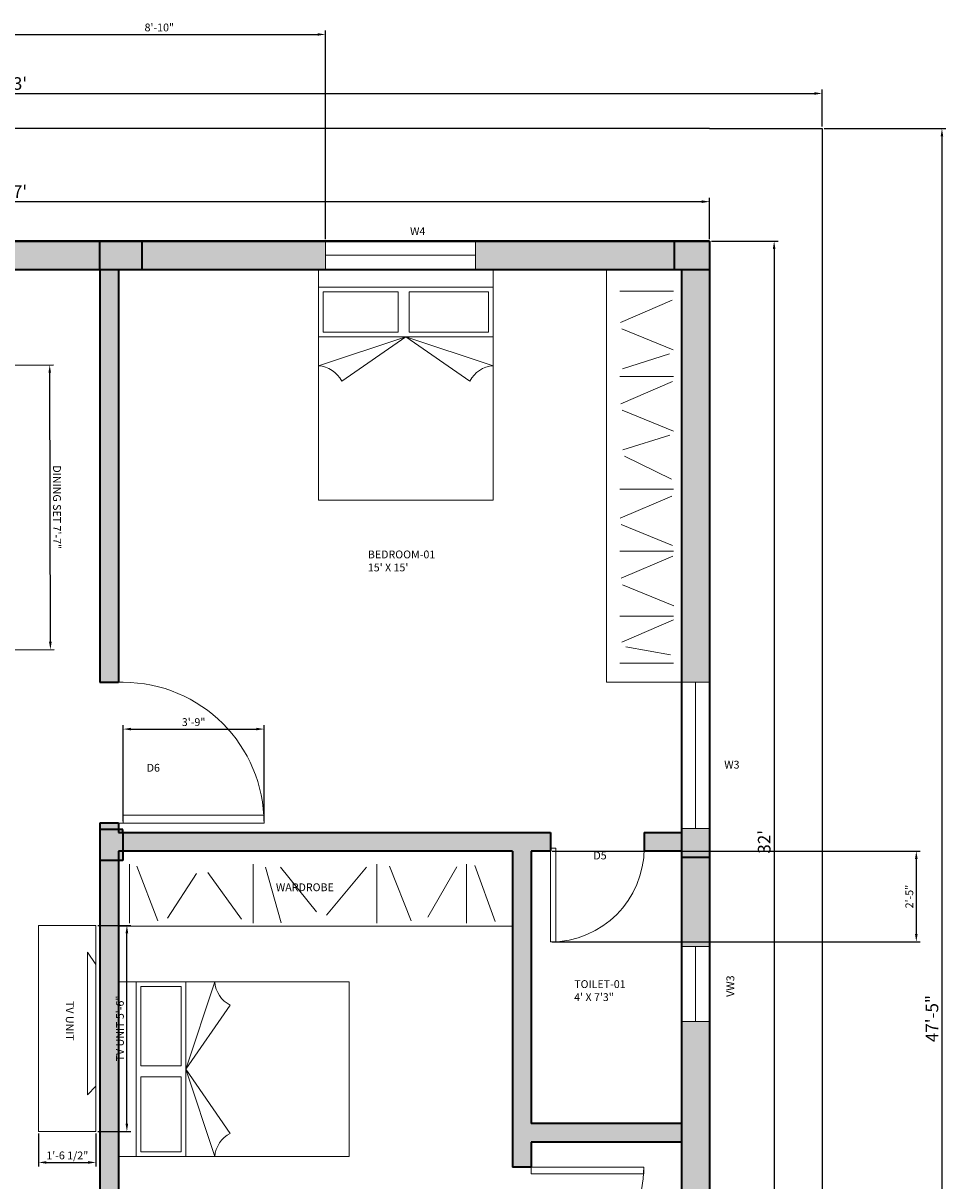
# Model space of a CAD drawing. Units: inches. Extents: x 5395 to 6469, y -203 to 448.
# Tile 5 of 7: x 5715 to 6010, y 78 to 448. Entities that reach past the tile are written whole.
import ezdxf

# ---------------------------------------------------------------- set-up
doc = ezdxf.new("R2010")
doc.units = ezdxf.units.IN
for name, color, linetype, lineweight in [('A-ANNO-DIMS', 2, 'Continuous', 18), ('A-ANNO-TEXT', 6, 'Continuous', 18), ('A-AREA-IDEN', 6, 'Continuous', 18), ('A-COLS', 7, 'Continuous', 35), ('A-COLS-PATT', 2, 'Continuous', 13), ('A-EQPM', 70, 'Continuous', 18), ('A-FLOR-CASE', 32, 'Continuous', 18), ('A-GLAZ', 4, 'Continuous', 18), ('A-WALL', 7, 'Continuous', 35), ('A-WALL-PATT', 11, 'Continuous', 9), ('C-PROP', 7, 'Continuous', 25), ('door', 240, 'Continuous', 18), ('furniture', 70, 'Continuous', 18)]:
    doc.layers.add(name, color=color, linetype=linetype, lineweight=lineweight)
doc.styles.get("Standard").update_dxf_attribs({"font": 'arial.ttf'})
doc.dimstyles.new('ISO-25', dxfattribs={"dimtxt": 2.5, "dimasz": 2.5, "dimexe": 1.25, "dimexo": 0.625, "dimtad": 1, "dimdec": 1, "dimlunit": 3, "dimtxsty": 'Standard', "dimcen": 2.5, "dimadec": 0, "dimazin": 0, "dimtfac": 1, "dimtdec": 1, "dimtmove": 0, "dimatfit": 3, "dimfxl": 1, "dimarcsym": 0})

# ---------------------------------------------------------------- blocks, each defined once
blk = doc.blocks.new('*U4')
for p, q in [((0, 0), (0, 5)), ((30, 0), (30, 5))]:
    blk.add_line(p, q)
blk.add_lwpolyline([(0, 0), (0, -30), (1.75, -30), (1.75, 0)], close=True)
blk.add_arc((0, 0), 30, 270, 0)
blk = doc.blocks.new('*U5')
for p, q in [((-30, 0), (-30, 5)), ((0, 0), (0, 5))]:
    blk.add_line(p, q)
blk.add_lwpolyline([(0, 0), (0, -30), (-1.75, -30), (-1.75, 0)], close=True)
blk.add_arc((0, 0), 30, 180, 270)
blk = doc.blocks.new('modern bed')
for p, q in [((-55.85, 73.76), (-55.85, 0)), ((0, 0), (0, 73.76)), ((-55.85, 68.07), (0, 68.07)), ((-54.35, 66.57), (-54.35, 53.68)), ((-54.35, 66.57), (-30.33, 66.57)), ((-30.33, 66.57), (-30.33, 53.68)), ((-26.87, 66.57), (-1.5, 66.57)), ((-26.87, 66.57), (-26.87, 53.68)), ((-1.5, 53.68), (-1.5, 66.57)), ((-55.85, 52.18), (0, 52.18)), ((-27.93, 52.18), (-55.85, 42.95)), ((-54.35, 53.68), (-30.33, 53.68)), ((-27.93, 52.18), (-48.41, 38.03)), ((-27.93, 52.18), (0, 42.95)), ((-27.93, 52.18), (-7.44, 38.03)), ((-26.87, 53.68), (-1.5, 53.68)), ((-55.85, 0), (0, 0))]:
    blk.add_line(p, q)
blk.add_lwpolyline([(-55.85, 73.76), (0, 73.76)])
for centre, start, end in [((-56.5, 33.89), 27.0819, 85.9278), ((0.64, 33.89), 94.0722, 152.9181)]:
    blk.add_arc(centre, 9.08, start, end)
blk = doc.blocks.new('tv')
for p, q in [((18.34, 53.39), (15.62, 57.31)), ((15.62, 57.31), (15.62, 11.74)), ((15.62, 11.74), (18.34, 14.53))]:
    blk.add_line(p, q)
blk.add_lwpolyline([(18.34, 0), (0, 0), (0, 65.9), (18.34, 65.9)], close=True)
blk = doc.blocks.new('*D17')
at = {"layer": 'A-ANNO-DIMS', "color": 0, "lineweight": -2, "transparency": 16777216}
for p, q in [((5490.94, 378.93), (5490.94, 392.2)), ((5493.44, 390.95), (5932.44, 390.95)), ((5934.94, 378.93), (5934.94, 392.2))]:
    blk.add_line(p, q, dxfattribs=at)
at = {"layer": 'A-ANNO-DIMS', "color": 0, "transparency": 16777216}
for points in [[(5493.44, 391.36), (5493.44, 390.53), (5490.94, 390.95)], [(5932.44, 391.36), (5932.44, 390.53), (5934.94, 390.95)]]:
    blk.add_solid(points, dxfattribs=at)
at = {"layer": 'Defpoints', "color": 0, "transparency": 16777216}
for p in [(5934.94, 390.95), (5490.94, 378.31), (5934.94, 378.31)]:
    blk.add_point(p, dxfattribs=at)
at = {"layer": 'A-ANNO-DIMS', "color": 0, "transparency": 16777216, "insert": (5712.94, 393.61), "char_height": 4, "attachment_point": 5}
blk.add_mtext("37'", dxfattribs=at)
blk = doc.blocks.new('*D18')
at = {"layer": 'A-ANNO-DIMS', "color": 0, "lineweight": -2, "transparency": 16777216}
for p, q in [((5454.94, 414.93), (5454.94, 426.78)), ((5970.94, 414.93), (5970.94, 426.78)), ((5457.44, 425.53), (5968.44, 425.53))]:
    blk.add_line(p, q, dxfattribs=at)
at = {"layer": 'A-ANNO-DIMS', "color": 0, "transparency": 16777216}
for points in [[(5457.44, 425.95), (5457.44, 425.12), (5454.94, 425.53)], [(5968.44, 425.95), (5968.44, 425.12), (5970.94, 425.53)]]:
    blk.add_solid(points, dxfattribs=at)
at = {"layer": 'Defpoints', "color": 0, "transparency": 16777216}
for p in [(5970.94, 425.53), (5454.94, 414.31), (5970.94, 414.31)]:
    blk.add_point(p, dxfattribs=at)
at = {"layer": 'A-ANNO-DIMS', "color": 0, "transparency": 16777216, "insert": (5712.94, 428.2), "char_height": 4, "attachment_point": 5}
blk.add_mtext("43'", dxfattribs=at)
blk = doc.blocks.new('*D19')
at = {"layer": 'A-ANNO-DIMS', "color": 0, "lineweight": -2, "transparency": 16777216}
for p, q in [((5971.63, 414.31), (6010.49, 414.31)), ((6009.24, 411.81), (6009.24, -152.19)), ((5971.63, -154.69), (6010.49, -154.69))]:
    blk.add_line(p, q, dxfattribs=at)
at = {"layer": 'A-ANNO-DIMS', "color": 0, "transparency": 16777216}
for points in [[(6008.82, 411.81), (6009.65, 411.81), (6009.24, 414.31)], [(6008.82, -152.19), (6009.65, -152.19), (6009.24, -154.69)]]:
    blk.add_solid(points, dxfattribs=at)
at = {"layer": 'Defpoints', "color": 0, "transparency": 16777216}
for p in [(5971, 414.31), (5971, -154.69), (6009.24, -154.69)]:
    blk.add_point(p, dxfattribs=at)
at = {"layer": 'A-ANNO-DIMS', "color": 0, "transparency": 16777216, "insert": (6006.58, 129.81), "char_height": 4, "attachment_point": 5, "rotation": 90}
blk.add_mtext('47\'-5"', dxfattribs=at)
blk = doc.blocks.new('*D22')
at = {"layer": 'A-ANNO-DIMS', "color": 0, "lineweight": -2, "transparency": 16777216}
for p, q in [((5935.56, 378.31), (5956.84, 378.31)), ((5955.59, 375.81), (5955.59, -3.19)), ((5935.56, -5.69), (5956.84, -5.69))]:
    blk.add_line(p, q, dxfattribs=at)
at = {"layer": 'A-ANNO-DIMS', "color": 0, "transparency": 16777216}
for points in [[(5955.17, 375.81), (5956, 375.81), (5955.59, 378.31)], [(5955.17, -3.19), (5956, -3.19), (5955.59, -5.69)]]:
    blk.add_solid(points, dxfattribs=at)
at = {"layer": 'Defpoints', "color": 0, "transparency": 16777216}
for p in [(5934.94, 378.31), (5934.94, -5.69), (5955.59, -5.69)]:
    blk.add_point(p, dxfattribs=at)
at = {"layer": 'A-ANNO-DIMS', "color": 0, "transparency": 16777216, "insert": (5952.92, 186.31), "char_height": 4, "attachment_point": 5, "rotation": 90}
blk.add_mtext("32'", dxfattribs=at)
blk = doc.blocks.new('WINDOW-48IN')
for p, q in [((0, 0), (0, 9)), ((48, 0), (48, 9)), ((0, 4.5), (48, 4.5))]:
    blk.add_line(p, q)
blk = doc.blocks.new('WINDOW-24IN')
for p, q in [((0, 24), (9, 24)), ((4.5, 0), (4.5, 24)), ((0, 0), (9, 0))]:
    blk.add_line(p, q)
blk = doc.blocks.new('*D51')
at = {"layer": 'A-ANNO-DIMS', "color": 0, "lineweight": -2, "transparency": 16777216}
for p, q in [((5710.93, 338.72), (5725.21, 338.76)), ((5724.17, 250.25), (5723.96, 336.25)), ((5711.15, 247.72), (5725.43, 247.76))]:
    blk.add_line(p, q, dxfattribs=at)
at = {"layer": 'A-ANNO-DIMS', "color": 0, "transparency": 16777216}
for points in [[(5724.38, 336.25), (5723.55, 336.25), (5723.96, 338.75)], [(5724.59, 250.25), (5723.75, 250.25), (5724.18, 247.75)]]:
    blk.add_solid(points, dxfattribs=at)
at = {"layer": 'Defpoints', "color": 0, "transparency": 16777216}
for p in [(5710.31, 338.72), (5723.96, 338.75), (5710.53, 247.72)]:
    blk.add_point(p, dxfattribs=at)
at = {"layer": 'A-ANNO-DIMS', "color": 0, "transparency": 16777216, "insert": (5725.98, 293.26), "char_height": 2.5, "attachment_point": 5, "rotation": 270.1373}
blk.add_mtext('DINING SET 7\'-7"', dxfattribs=at)
blk = doc.blocks.new('*D57')
at = {"layer": 'A-ANNO-DIMS', "color": 0, "lineweight": -2, "transparency": 16777216}
for p, q in [((5739.38, 159.6), (5749.89, 159.6)), ((5748.64, 96.2), (5748.64, 157.1)), ((5739.38, 93.7), (5749.89, 93.7))]:
    blk.add_line(p, q, dxfattribs=at)
at = {"layer": 'A-ANNO-DIMS', "color": 0, "transparency": 16777216}
for points in [[(5748.22, 157.1), (5749.05, 157.1), (5748.64, 159.6)], [(5748.22, 96.2), (5749.05, 96.2), (5748.64, 93.7)]]:
    blk.add_solid(points, dxfattribs=at)
at = {"layer": 'Defpoints', "color": 0, "transparency": 16777216}
for p in [(5738.75, 159.6), (5748.64, 159.6), (5738.75, 93.7)]:
    blk.add_point(p, dxfattribs=at)
at = {"layer": 'A-ANNO-DIMS', "color": 0, "transparency": 16777216, "insert": (5746.74, 126.65), "char_height": 2.5, "attachment_point": 5, "rotation": 90}
blk.add_mtext('TV UNIT 5\'-6"', dxfattribs=at)
blk = doc.blocks.new('*D58')
at = {"layer": 'A-ANNO-DIMS', "color": 0, "lineweight": -2, "transparency": 16777216}
for p, q in [((5720.41, 93.08), (5720.41, 82.57)), ((5738.75, 93.08), (5738.75, 82.57)), ((5722.91, 83.82), (5736.25, 83.82))]:
    blk.add_line(p, q, dxfattribs=at)
at = {"layer": 'A-ANNO-DIMS', "color": 0, "transparency": 16777216}
for points in [[(5722.91, 84.24), (5722.91, 83.4), (5720.41, 83.82)], [(5736.25, 84.24), (5736.25, 83.4), (5738.75, 83.82)]]:
    blk.add_solid(points, dxfattribs=at)
at = {"layer": 'Defpoints', "color": 0, "transparency": 16777216}
for p in [(5720.41, 93.7), (5738.75, 93.7), (5738.75, 83.82)]:
    blk.add_point(p, dxfattribs=at)
at = {"layer": 'A-ANNO-DIMS', "color": 0, "transparency": 16777216, "insert": (5729.58, 85.74), "char_height": 2.5, "attachment_point": 5}
blk.add_mtext('1\'-6 1/2"', dxfattribs=at)
blk = doc.blocks.new('*D63')
at = {"layer": 'A-ANNO-DIMS', "color": 0, "lineweight": -2, "transparency": 16777216}
for p, q in [((5705.93, 378.93), (5705.93, 445.66)), ((5708.43, 444.41), (5809.6, 444.41)), ((5812.1, 378.93), (5812.1, 445.66))]:
    blk.add_line(p, q, dxfattribs=at)
at = {"layer": 'A-ANNO-DIMS', "color": 0, "transparency": 16777216}
for points in [[(5708.43, 444.82), (5708.43, 443.99), (5705.93, 444.41)], [(5809.6, 444.82), (5809.6, 443.99), (5812.1, 444.41)]]:
    blk.add_solid(points, dxfattribs=at)
at = {"layer": 'Defpoints', "color": 0, "transparency": 16777216}
for p in [(5812.1, 444.41), (5705.93, 378.31), (5812.1, 378.31)]:
    blk.add_point(p, dxfattribs=at)
at = {"layer": 'A-ANNO-DIMS', "color": 0, "transparency": 16777216, "insert": (5759.01, 446.31), "char_height": 2.5, "attachment_point": 5}
blk.add_mtext('8\'-10"', dxfattribs=at)
blk = doc.blocks.new('*D70')
at = {"layer": 'A-ANNO-DIMS', "color": 0, "lineweight": -2, "transparency": 16777216}
for p, q in [((5747.44, 192.88), (5747.44, 223.6)), ((5749.94, 222.35), (5790, 222.35)), ((5792.5, 192.88), (5792.5, 223.6))]:
    blk.add_line(p, q, dxfattribs=at)
at = {"layer": 'A-ANNO-DIMS', "color": 0, "transparency": 16777216}
for points in [[(5749.94, 222.77), (5749.94, 221.94), (5747.44, 222.35)], [(5790, 222.77), (5790, 221.94), (5792.5, 222.35)]]:
    blk.add_solid(points, dxfattribs=at)
at = {"layer": 'Defpoints', "color": 0, "transparency": 16777216}
for p in [(5792.5, 222.35), (5747.44, 192.25), (5792.5, 192.25)]:
    blk.add_point(p, dxfattribs=at)
at = {"layer": 'A-ANNO-DIMS', "color": 0, "transparency": 16777216, "insert": (5769.97, 224.26), "char_height": 2.5, "attachment_point": 5}
blk.add_mtext('3\'-9"', dxfattribs=at)
blk = doc.blocks.new('*D71')
at = {"layer": 'A-ANNO-DIMS', "color": 0, "lineweight": -2, "transparency": 16777216}
for p, q in [((5884.66, 183.31), (6002.29, 183.31)), ((6001.04, 180.81), (6001.04, 156.81)), ((5884.66, 154.31), (6002.29, 154.31))]:
    blk.add_line(p, q, dxfattribs=at)
at = {"layer": 'A-ANNO-DIMS', "color": 0, "transparency": 16777216}
for points in [[(6000.62, 180.81), (6001.45, 180.81), (6001.04, 183.31)], [(6000.62, 156.81), (6001.45, 156.81), (6001.04, 154.31)]]:
    blk.add_solid(points, dxfattribs=at)
at = {"layer": 'Defpoints', "color": 0, "transparency": 16777216}
for p in [(5884.03, 183.31), (5884.03, 154.31), (6001.04, 154.31)]:
    blk.add_point(p, dxfattribs=at)
at = {"layer": 'A-ANNO-DIMS', "color": 0, "transparency": 16777216, "insert": (5999.13, 168.81), "char_height": 2.5, "attachment_point": 5, "rotation": 90}
blk.add_mtext('2\'-5"', dxfattribs=at)

msp = doc.modelspace()

# ---------------------------------------------------------------- hatches: boundary and pattern name
at = {"layer": 'A-COLS-PATT'}
h = msp.add_hatch(color=256, dxfattribs=at)
h.dxf.hatch_style = 1
h.paths.add_polyline_path([(5627.19, 378.31), (5619.94, 378.31), (5619.94, 369.31), (5619.94, 367.55), (5627.19, 367.55), (5627.19, 369.31)])
h.paths.add_polyline_path([(5753.55, 378.31), (5739.94, 378.31), (5739.94, 369.31), (5753.55, 369.31)])
h.paths.add_polyline_path([(5934.94, 378.31), (5923.7, 378.31), (5923.7, 369.31), (5925.94, 369.31), (5934.94, 369.31)])
h = msp.add_hatch(color=256, dxfattribs=at)
h.dxf.hatch_style = 1
h.paths.add_polyline_path([(5747.34, 189.31), (5745.94, 189.31), (5745.94, 190.23), (5739.94, 190.23), (5739.94, 180.33), (5745.94, 180.33), (5745.94, 183.31), (5747.34, 183.31)])
h.paths.add_polyline_path([(5747.34, 190.23), (5745.94, 190.23), (5745.94, 189.31), (5747.34, 189.31)], flags=17)
h.paths.add_polyline_path([(5747.34, 183.31), (5745.94, 183.31), (5745.94, 180.33), (5747.34, 180.33)], flags=17)
h = msp.add_hatch(color=256, dxfattribs=at)
h.dxf.hatch_style = 1
h.paths.add_polyline_path([(5934.94, 190.61), (5925.94, 190.61), (5925.94, 181.4), (5934.94, 181.4)])
at = {"layer": 'A-WALL-PATT'}
h = msp.add_hatch(color=256, dxfattribs=at)
h.dxf.hatch_style = 1
h.paths.add_polyline_path([(5538.88, 378.31), (5499.94, 378.31), (5499.94, 369.31), (5538.88, 369.31)])
h.paths.add_polyline_path([(5499.94, 276.14), (5490.94, 276.14), (5490.94, 227.71), (5499.94, 227.71), (5499.94, 237.31)])
h.paths.add_polyline_path([(5565.94, 243.31), (5499.94, 243.31), (5499.94, 237.31), (5559.94, 237.31), (5559.94, 225.31), (5565.94, 225.31)])
h.paths.add_polyline_path([(5625.94, 367.55), (5619.94, 367.55), (5619.94, 237.31), (5625.94, 237.31)])
h.paths.add_polyline_path([(5745.94, 369.31), (5739.94, 369.31), (5739.94, 237.31), (5745.94, 237.31)])
h.paths.add_polyline_path([(5745.94, 192.25), (5739.94, 192.25), (5739.94, 190.23), (5745.94, 190.23)])
h.paths.add_polyline_path([(5745.94, 180.33), (5739.94, 180.33), (5739.94, 47.04), (5745.94, 47.04)])
h.paths.add_polyline_path([(5877.94, 183.31), (5884.03, 183.31), (5884.03, 189.31), (5747.34, 189.31), (5747.34, 183.31), (5871.94, 183.31), (5871.94, 82.27), (5877.94, 82.27), (5877.94, 90.31), (5925.94, 90.31), (5925.94, 96.31), (5877.94, 96.31)])
h.paths.add_polyline_path([(5934.94, 128.85), (5925.94, 128.85), (5925.94, 55.61), (5934.94, 55.61)])
h.paths.add_polyline_path([(5934.94, 181.4), (5925.94, 181.4), (5925.94, 152.85), (5934.94, 152.85)])
h.paths.add_polyline_path([(5925.94, 189.31), (5914.03, 189.31), (5914.03, 183.31), (5925.94, 183.31)], flags=17)
h.paths.add_polyline_path([(5934.94, 369.31), (5925.94, 369.31), (5925.94, 237.31), (5934.94, 237.31)])
h.paths.add_polyline_path([(5657.93, 378.31), (5627.19, 378.31), (5627.19, 369.31), (5657.93, 369.31)])
h.paths.add_polyline_path([(5619.94, 378.31), (5586.88, 378.31), (5586.88, 369.31), (5619.94, 369.31)])
h.paths.add_polyline_path([(5739.94, 378.31), (5705.93, 378.31), (5705.93, 369.31), (5739.94, 369.31)])
h.paths.add_polyline_path([(5812.1, 378.31), (5753.55, 378.31), (5753.55, 369.31), (5812.1, 369.31)])
h.paths.add_polyline_path([(5923.7, 378.31), (5860.1, 378.31), (5860.1, 369.31), (5923.7, 369.31)])
h.paths.add_polyline_path([(5499.94, 203.71), (5490.94, 203.71), (5490.94, 189.31), (5499.94, 189.31)])
h.paths.add_polyline_path([(5612.93, 189.31), (5499.94, 189.31), (5499.94, 183.31), (5612.93, 183.31)])
h.paths.add_polyline_path([(5499.94, 178.42), (5490.94, 178.42), (5490.94, 132.59), (5499.94, 132.59)])
h.paths.add_polyline_path([(5499.94, 84.59), (5490.94, 84.59), (5490.94, 47.04), (5499.94, 47.04)])
h.paths.add_polyline_path([(5499.94, 11.04), (5490.94, 11.04), (5490.94, 3.31), (5499.94, 3.31)])
h.paths.add_polyline_path([(5532.25, 3.31), (5502.78, 3.31), (5502.78, -5.69), (5532.25, -5.69)])
h.paths.add_polyline_path([(5601.84, 3.31), (5580.25, 3.31), (5580.25, -5.69), (5601.84, -5.69)])
h.paths.add_polyline_path([(5625.94, 3.31), (5614.13, 3.31), (5614.13, -5.69), (5625.94, -5.69)])
h.paths.add_polyline_path([(5787.9, 3.31), (5748.46, 3.31), (5748.46, -5.69), (5787.9, -5.69)])
h.paths.add_polyline_path([(5737.31, 3.31), (5697.94, 3.31), (5697.94, -5.69), (5737.31, -5.69)])
h.paths.add_polyline_path([(5745.94, 11.04), (5739.94, 11.04), (5739.94, 3.31), (5745.94, 3.31)])
h.paths.add_polyline_path([(5922.21, 3.31), (5877.94, 3.31), (5877.94, 46.27), (5871.94, 46.27), (5871.94, 3.31), (5835.9, 3.31), (5835.9, -5.69), (5922.21, -5.69)])
h.paths.add_polyline_path([(5934.94, 31.61), (5925.94, 31.61), (5925.94, 3.31), (5934.94, 3.31)])

# ---------------------------------------------------------------- linework, layer by layer
at = {"layer": 'A-COLS'}
for p, q in [((5739.94, 369.31), (5739.94, 378.31)), ((5753.55, 369.31), (5753.55, 378.31)), ((5923.7, 369.31), (5923.7, 378.31)), ((5925.94, 369.31), (5934.94, 369.31)), ((5747.34, 190.23), (5739.94, 190.23)), ((5747.34, 189.31), (5747.34, 190.23)), ((5747.34, 189.31), (5747.34, 180.33)), ((5925.94, 181.4), (5934.94, 181.4)), ((5747.34, 180.33), (5739.94, 180.33))]:
    msp.add_line(p, q, dxfattribs=at)
at = {"layer": 'A-FLOR-CASE'}
for p, q in [((5901.94, 369.31), (5901.94, 237.31)), ((5906.22, 362.32), (5923.38, 362.32)), ((5906.48, 352.32), (5923, 359.42)), ((5906.87, 350.28), (5923.29, 343.58)), ((5922.13, 342.32), (5907.06, 337.56)), ((5906.22, 335.03), (5923.38, 335.03)), ((5906.61, 326.36), (5923.13, 333.45)), ((5906.99, 324.32), (5923.42, 317.62)), ((5922.26, 316.35), (5907.19, 311.59)), ((5907.73, 309.6), (5922.75, 302.28)), ((5906.22, 299.05), (5923.38, 299.05)), ((5906.31, 289.75), (5922.84, 296.84)), ((5906.7, 287.71), (5923.13, 281)), ((5906.22, 279.18), (5923.38, 279.18)), ((5906.7, 270.54), (5923.23, 277.63)), ((5907.09, 268.5), (5923.52, 261.8)), ((5906.22, 258.47), (5923.38, 258.47)), ((5906.84, 250.13), (5923.36, 257.22)), ((5908.12, 248.63), (5922.45, 246.07)), ((5906.22, 243.43), (5923.38, 243.43)), ((5925.94, 237.31), (5901.94, 237.31)), ((5749.45, 179.15), (5749.45, 160.34)), ((5751.85, 178.53), (5758.58, 161.04)), ((5789.04, 179.15), (5789.04, 160.34)), ((5792.91, 178.19), (5797.95, 160.37)), ((5809.23, 163.9), (5797.79, 178.19)), ((5825.22, 178.19), (5812.43, 162.89)), ((5828.58, 179.15), (5828.58, 160.34)), ((5832.62, 178.53), (5839.52, 161.04)), ((5854.16, 178.36), (5844.9, 162.22)), ((5857.19, 179.15), (5857.19, 160.34)), ((5859.88, 178.7), (5866.44, 160.87)), ((5761.59, 161.89), (5770.85, 176.19)), ((5774.55, 176.52), (5785.32, 161.56)), ((5871.94, 159.31), (5745.94, 159.31))]:
    msp.add_line(p, q, dxfattribs=at)
at = {"layer": 'A-GLAZ'}
for p, q in [((5925.94, 237.31), (5934.94, 237.31)), ((5930.44, 237.31), (5930.44, 190.61)), ((5925.94, 190.61), (5934.94, 190.61))]:
    msp.add_line(p, q, dxfattribs=at)
at = {"layer": 'A-WALL'}
for p, q in [((5490.94, 378.31), (5934.94, 378.31)), ((5490.94, 378.31), (5934.94, 378.31)), ((5934.94, 378.31), (5490.94, 378.31)), ((5934.94, 378.31), (5934.94, -5.69)), ((5627.19, 369.31), (5925.94, 369.31)), ((5739.94, 369.31), (5739.94, 237.31)), ((5745.94, 369.31), (5745.94, 237.31)), ((5925.94, 369.31), (5925.94, 3.31)), ((5739.94, 237.31), (5745.94, 237.31)), ((5745.94, 192.25), (5739.94, 192.25)), ((5739.94, 192.25), (5739.94, 47.04)), ((5745.94, 192.25), (5745.94, 189.31)), ((5745.94, 189.31), (5884.03, 189.31)), ((5884.03, 189.31), (5884.03, 183.31)), ((5914.03, 189.31), (5914.03, 183.31)), ((5914.03, 189.31), (5925.94, 189.31)), ((5745.94, 183.31), (5745.94, 47.04)), ((5871.94, 183.31), (5745.94, 183.31)), ((5871.94, 183.31), (5871.94, 82.27)), ((5877.94, 183.31), (5877.94, 96.31)), ((5884.03, 183.31), (5877.94, 183.31)), ((5925.94, 183.31), (5914.03, 183.31)), ((5925.94, 96.31), (5877.94, 96.31)), ((5925.94, 90.31), (5877.94, 90.31)), ((5877.94, 90.31), (5877.94, 82.27)), ((5877.94, 82.27), (5871.94, 82.27))]:
    msp.add_line(p, q, dxfattribs=at)
at = {"layer": 'C-PROP'}
for p, q in [((5934.94, 414.31), (5490.94, 414.31)), ((5934.94, 414.31), (5970.94, 414.31)), ((5970.94, 414.31), (5970.94, -154.69))]:
    msp.add_line(p, q, dxfattribs=at)

# ---------------------------------------------------------------- block references
at = {"layer": 'A-EQPM'}
msp.add_blockref('tv', (5720.41, 93.7), dxfattribs=at)
at = {"layer": 'A-GLAZ'}
for name, p in [('WINDOW-48IN', (5812.1, 369.31)), ('WINDOW-24IN', (5925.94, 128.85))]:
    msp.add_blockref(name, p, dxfattribs=at)
at = {"layer": 'door', "rotation": 90}
for name, p, xscale, yscale, zscale in [('*U4', (5747.44, 192.25), 1.501711826160258, 1.501711826160258, 1.501711826160258), ('*U5', (5877.94, 82.27), 1.199999999999999, 1.199999999999999, 1.199999999999999)]:
    msp.add_blockref(name, p, dxfattribs=dict(at, xscale=xscale, yscale=yscale, zscale=zscale))
at = {"layer": 'door'}
msp.add_blockref('*U4', (5884.03, 184.31), dxfattribs=at)
at = {"layer": 'furniture'}
msp.add_blockref('modern bed', (5865.74, 295.54), dxfattribs=at)
at = {"layer": 'furniture', "rotation": 90}
msp.add_blockref('modern bed', (5819.7, 141.53), dxfattribs=at)

# ---------------------------------------------------------------- texts
at = {"layer": 'A-ANNO-TEXT', "char_height": 2.5, "attachment_point": 1}
for s, insert in [('W4', (5839.18, 382.74)), ('D6', (5754.97, 211.24)), ('W3', (5939.63, 212.22)), ('D5', (5897.8, 183.19))]:
    msp.add_mtext_dynamic_manual_height_columns(s, width=62.1492, gutter_width=12.5, heights=[0], dxfattribs=dict(at, insert=insert))
for s, insert, rotation in [('VW3', (5940.33, 136.75), 90), ('TV UNIT', (5731.63, 135.45), 270)]:
    msp.add_mtext_dynamic_manual_height_columns(s, width=62.1492, gutter_width=12.5, heights=[0], dxfattribs=dict(at, insert=insert, rotation=rotation))
at = {"layer": 'A-AREA-IDEN', "char_height": 2.5, "attachment_point": 1}
for s, insert in [("BEDROOM-01\\P15' X 15'", (5825.68, 279.43)), ('WARDROBE\\P ', (5796.28, 173.03)), ('TOILET-01\\P4\' X 7\'3"', (5891.66, 142.08))]:
    msp.add_mtext_dynamic_manual_height_columns(s, width=62.1492, gutter_width=12.5, heights=[0], dxfattribs=dict(at, insert=insert))

# ---------------------------------------------------------------- dimensions: what is measured, and where the dimension line sits
at = {"layer": 'A-ANNO-DIMS'}
for base, p1, p2, override, picture, middle in [((5812.1, 444.41), (5705.93, 378.31), (5812.1, 378.31), {"dimdec": 1, "dimlfac": 1, "dimrnd": 0, "dimzin": 1, "dimdsep": 46, "dimlunit": 4, "dimfrac": 2}, '*D63', (5759.01, 446.31)), ((5934.94, 390.95), (5490.94, 378.31), (5934.94, 378.31), {"dimtxt": 4, "dimclrd": 0, "dimclre": 0, "dimclrt": 0}, '*D17', (5712.94, 393.61)), ((5792.5, 222.35), (5747.44, 192.25), (5792.5, 192.25), {"dimdec": 1, "dimlfac": 1, "dimrnd": 0, "dimzin": 1, "dimdsep": 46, "dimlunit": 4, "dimfrac": 2}, '*D70', (5769.97, 224.26)), ((5738.75, 83.82), (5720.41, 93.7), (5738.75, 93.7), {"dimdec": 1, "dimlfac": 1, "dimrnd": 0, "dimzin": 1, "dimdsep": 46, "dimlunit": 4, "dimfrac": 2}, '*D58', (5729.58, 85.74))]:
    dim = msp.add_linear_dim(base=base, p1=p1, p2=p2, dimstyle='ISO-25', override=override, dxfattribs=at)
    dim.commit()
    dim.dimension.update_dxf_attribs({"geometry": picture, "text_midpoint": middle})
for p1, p2, distance, picture, middle in [((5454.94, 414.31), (5970.94, 414.31), 11.23, '*D18', (5712.94, 428.2)), ((5971, 414.31), (5971, -154.69), 38.23, '*D19', (6006.58, 129.81))]:
    dim = msp.add_aligned_dim(p1=p1, p2=p2, distance=distance, dimstyle='ISO-25', override={"dimtxt": 4, "dimclrd": 0, "dimclre": 0, "dimclrt": 0}, dxfattribs=at)
    dim.commit()
    dim.dimension.update_dxf_attribs({"geometry": picture, "text_midpoint": middle})
for base, p1, p2, override, picture, middle in [((5955.59, -5.69), (5934.94, 378.31), (5934.94, -5.69), {"dimtxt": 4, "dimclrd": 0, "dimclre": 0, "dimclrt": 0}, '*D22', (5952.92, 186.31)), ((6001.04, 154.31), (5884.03, 183.31), (5884.03, 154.31), {"dimdec": 1, "dimlfac": 1, "dimrnd": 0, "dimzin": 1, "dimdsep": 46, "dimlunit": 4, "dimfrac": 2}, '*D71', (5999.13, 168.81))]:
    dim = msp.add_linear_dim(base=base, p1=p1, p2=p2, angle=90, dimstyle='ISO-25', override=override, dxfattribs=at)
    dim.commit()
    dim.dimension.update_dxf_attribs({"geometry": picture, "text_midpoint": middle})
for base, p1, p2, angle, text, picture, middle in [((5723.96, 338.75), (5710.53, 247.72), (5710.31, 338.72), 90.1373, 'DINING SET <>', '*D51', (5725.98, 293.26)), ((5748.64, 159.6), (5738.75, 93.7), (5738.75, 159.6), 90, 'TV UNIT <>', '*D57', (5746.74, 126.65))]:
    dim = msp.add_linear_dim(base=base, p1=p1, p2=p2, angle=angle, text=text, dimstyle='ISO-25', override={"dimdec": 1, "dimlfac": 1, "dimrnd": 0, "dimzin": 1, "dimdsep": 46, "dimlunit": 4, "dimfrac": 2}, dxfattribs=at)
    dim.commit()
    dim.dimension.update_dxf_attribs({"geometry": picture, "text_midpoint": middle})

doc.saveas('drawing.dxf')
